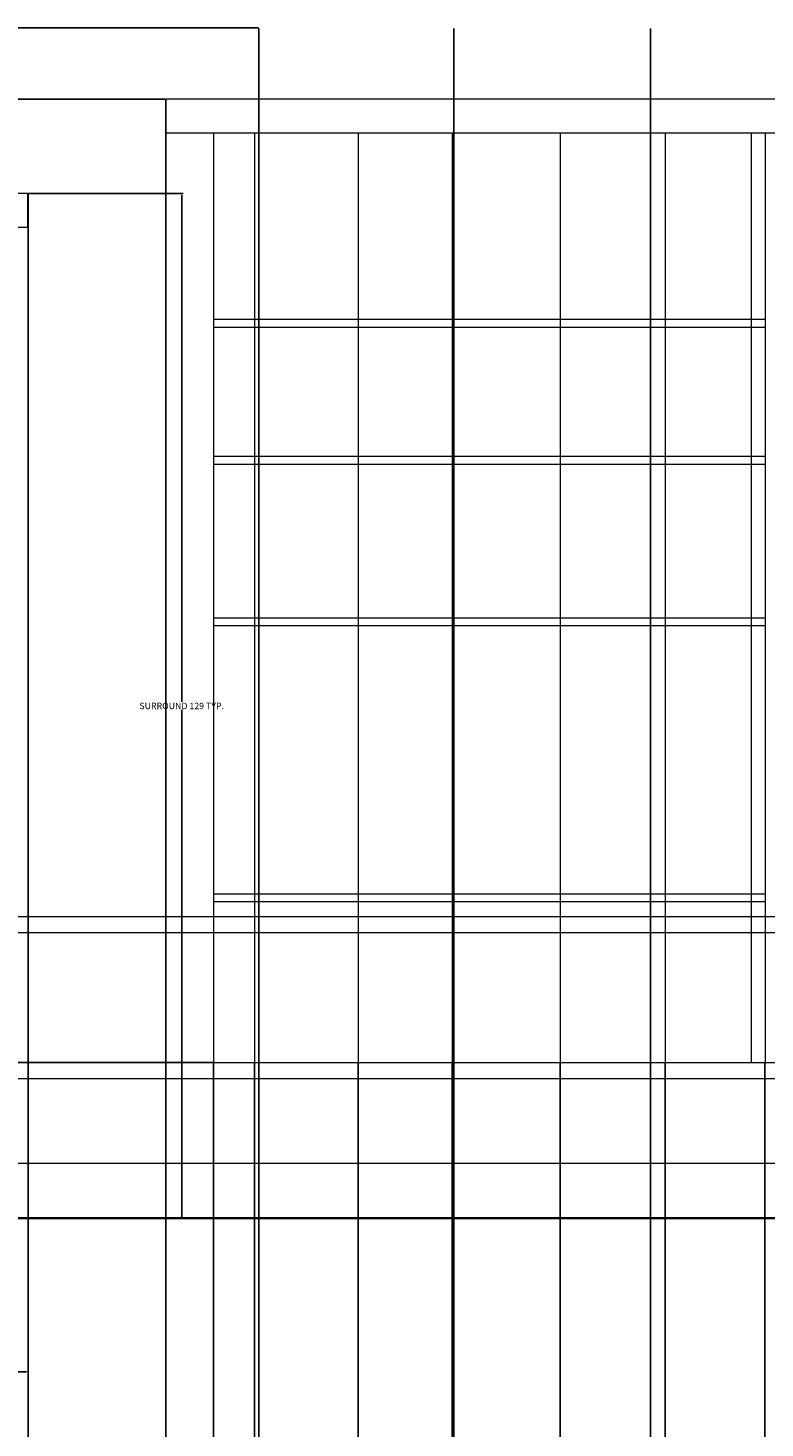
# Model space of a CAD drawing. Units: inches. Extents: x 69 to 650, y -16 to 573.
# Tile 14 of 26: x 290 to 383, y 218 to 394. Entities that reach past the tile are written whole.
import ezdxf

# ---------------------------------------------------------------- set-up
doc = ezdxf.new("R2010")
doc.units = ezdxf.units.IN
doc.header["$MEASUREMENT"] = 0
for name, color, linetype, lineweight in [('A-ANNO-DIMS', 2, 'Continuous', 18), ('A-ELEV', 8, 'Continuous', 18), ('A-GLAZ', 4, 'Continuous', 18), ('A-WALL', 7, 'Continuous', 35)]:
    doc.layers.add(name, color=color, linetype=linetype, lineweight=lineweight)
doc.styles.get("Standard").update_dxf_attribs({"font": 'arial.ttf'})
doc.dimstyles.get("Standard").update_dxf_attribs({"dimtxt": 0.8125, "dimasz": 0.18, "dimexe": 0.18, "dimexo": 0.0625, "dimgap": 0.09, "dimtad": 0, "dimtih": 1, "dimtoh": 1, "dimdec": 4, "dimzin": 0, "dimdsep": 46, "dimlunit": 4, "dimtxsty": 'Standard', "dimcen": 0.09, "dimadec": 0, "dimazin": 0, "dimtfac": 1, "dimtdec": 4, "dimtofl": 0, "dimtmove": 0, "dimatfit": 3, "dimfxl": 1, "dimtolj": 1, "dimtzin": 0, "dimarcsym": 0})

# ---------------------------------------------------------------- blocks, each defined once
blk = doc.blocks.new('WIN-ARCH-SURROUND')
for p, q in [((0, 129.06), (0, 124.83)), ((82.63, 129.06), (0, 129.06)), ((82.63, 124.83), (82.63, 129.06)), ((0, 124.83), (82.63, 124.83)), ((2.69, 109.21), (2.69, 124.83)), ((79.05, 109.21), (79.05, 124.83)), ((3.69, 109.21), (2.69, 109.21)), ((3.69, 109.21), (3.69, 105.89)), ((3.69, 109.21), (78.05, 109.21)), ((7.69, 109.21), (7.69, 105.89)), ((8.73, 105.89), (8.73, 109.21)), ((38.31, 109.21), (38.31, 38)), ((40.31, 109.21), (40.31, 38)), ((74.05, 109.21), (74.05, 105.89)), ((78.05, 109.21), (79.05, 109.21)), ((78.05, 109.21), (78.05, 105.89)), ((3.69, 92.64), (3.69, 87.15)), ((7.69, 92.64), (7.69, 87.15)), ((74.05, 92.64), (74.05, 87.15)), ((78.05, 92.64), (78.05, 87.15)), ((3.69, 73.9), (3.69, 69.84)), ((7.69, 73.9), (7.69, 69.84)), ((74.05, 73.9), (74.05, 69.84)), ((78.05, 73.9), (78.05, 69.84)), ((3.69, 56.59), (3.69, 51.51)), ((7.69, 56.59), (7.69, 51.51)), ((74.05, 56.59), (74.05, 51.51)), ((78.05, 56.59), (78.05, 51.51)), ((3.69, 38.26), (3.69, 33.16)), ((7.69, 38.26), (7.69, 33.16)), ((74.05, 38.26), (74.05, 33.16)), ((78.05, 38.26), (78.05, 33.16)), ((3.69, 19.91), (3.69, 0)), ((7.69, 19.91), (7.69, 0)), ((74.05, 19.91), (74.05, 0)), ((78.05, 19.91), (78.05, 0))]:
    blk.add_line(p, q)
for points in [[(8.73, 109.21), (73.05, 109.21), (73.05, 38.26), (8.73, 38.26)], [(9.73, 108.21), (72.05, 108.21), (72.05, 39.26), (9.73, 39.26)], [(2.69, 105.89), (8.73, 105.89), (8.73, 92.64), (2.69, 92.64)], [(73.05, 105.89), (79.1, 105.89), (79.1, 92.64), (73.05, 92.64)], [(2.69, 87.15), (8.73, 87.15), (8.73, 73.9), (2.69, 73.9)], [(73.05, 87.15), (79.1, 87.15), (79.1, 73.9), (73.05, 73.9)], [(2.69, 69.84), (8.73, 69.84), (8.73, 56.59), (2.69, 56.59)], [(73.05, 69.84), (79.1, 69.84), (79.1, 56.59), (73.05, 56.59)], [(2.69, 51.51), (8.73, 51.51), (8.73, 38.26), (2.69, 38.26)], [(73.05, 51.51), (79.1, 51.51), (79.1, 38.26), (73.05, 38.26)], [(2.65, 33.16), (8.69, 33.16), (8.69, 19.91), (2.65, 19.91)], [(73.01, 33.16), (79.06, 33.16), (79.06, 19.91), (73.01, 19.91)]]:
    blk.add_lwpolyline(points, close=True)
blk.add_ellipse((40.89, 109.21), major_axis=(32.16, 0), ratio=0.165597, start_param=6.283185, end_param=9.424778)
blk = doc.blocks.new('*D13')
at = {"layer": 'A-ANNO-DIMS', "color": 0, "lineweight": -2, "transparency": 16777216}
for p, q in [((290.51, 372.99), (309.99, 372.99)), ((309.81, 372.81), (309.81, 308.97)), ((309.81, 244.11), (309.81, 307.95)), ((290.51, 243.93), (309.99, 243.93))]:
    blk.add_line(p, q, dxfattribs=at)
at = {"layer": 'A-ANNO-DIMS', "color": 0, "transparency": 16777216}
for points in [[(309.78, 372.81), (309.84, 372.81), (309.81, 372.99)], [(309.78, 244.11), (309.84, 244.11), (309.81, 243.93)]]:
    blk.add_solid(points, dxfattribs=at)
at = {"layer": 'Defpoints', "color": 0, "transparency": 16777216}
for p in [(290.45, 372.99), (309.81, 372.99), (290.45, 243.93)]:
    blk.add_point(p, dxfattribs=at)
at = {"layer": 'A-ANNO-DIMS', "color": 0, "transparency": 16777216, "insert": (309.81, 308.46), "char_height": 0.8125, "attachment_point": 5}
blk.add_mtext('\\A1;SURROUND 129 TYP.', dxfattribs=at)
blk = doc.blocks.new('*D14')
at = {"layer": 'A-ANNO-DIMS', "color": 0, "lineweight": -2, "transparency": 16777216}
for p, q in [((207.81, 243.87), (207.81, 224.39)), ((290.45, 243.87), (290.45, 224.39)), ((207.99, 224.57), (247.06, 224.57)), ((290.27, 224.57), (251.2, 224.57))]:
    blk.add_line(p, q, dxfattribs=at)
at = {"layer": 'A-ANNO-DIMS', "color": 0, "transparency": 16777216}
for points in [[(207.99, 224.6), (207.99, 224.54), (207.81, 224.57)], [(290.27, 224.6), (290.27, 224.54), (290.45, 224.57)]]:
    blk.add_solid(points, dxfattribs=at)
at = {"layer": 'Defpoints', "color": 0, "transparency": 16777216}
for p in [(207.81, 243.93), (290.45, 243.93), (290.45, 224.57)]:
    blk.add_point(p, dxfattribs=at)
at = {"layer": 'A-ANNO-DIMS', "color": 0, "transparency": 16777216, "insert": (249.13, 224.57), "char_height": 0.8125, "attachment_point": 5}
blk.add_mtext('\\A1;83 TYP.', dxfattribs=at)
blk = doc.blocks.new('*D19')
at = {"layer": 'A-ANNO-DIMS', "color": 0, "lineweight": -2, "transparency": 16777216}
for p, q in [((99.56, 471.72), (99.56, 572.74)), ((99.74, 572.56), (358.57, 572.56)), ((619.38, 572.56), (360.54, 572.56)), ((619.56, 87.99), (619.56, 572.74))]:
    blk.add_line(p, q, dxfattribs=at)
at = {"layer": 'A-ANNO-DIMS', "color": 0, "transparency": 16777216}
for points in [[(99.74, 572.59), (99.74, 572.53), (99.56, 572.56)], [(619.38, 572.59), (619.38, 572.53), (619.56, 572.56)]]:
    blk.add_solid(points, dxfattribs=at)
at = {"layer": 'Defpoints', "color": 0, "transparency": 16777216}
for p in [(619.56, 572.56), (99.56, 471.66), (619.56, 87.93)]:
    blk.add_point(p, dxfattribs=at)
at = {"layer": 'A-ANNO-DIMS', "color": 0, "transparency": 16777216, "insert": (359.56, 572.56), "char_height": 0.812, "attachment_point": 5}
blk.add_mtext('\\A1;520', dxfattribs=at)
blk = doc.blocks.new('*D25')
at = {"layer": 'A-ANNO-DIMS', "color": 0, "lineweight": -2, "transparency": 16777216}
for p, q in [((99.49, 243.93), (70.98, 243.93)), ((71.16, 243.75), (71.16, 228.3)), ((71.16, 211.83), (71.16, 227.29)), ((441.88, 211.65), (70.98, 211.65))]:
    blk.add_line(p, q, dxfattribs=at)
at = {"layer": 'A-ANNO-DIMS', "color": 0, "transparency": 16777216}
for points in [[(71.13, 243.75), (71.19, 243.75), (71.16, 243.93)], [(71.13, 211.83), (71.19, 211.83), (71.16, 211.65)]]:
    blk.add_solid(points, dxfattribs=at)
at = {"layer": 'Defpoints', "color": 0, "transparency": 16777216}
for p in [(71.16, 243.93), (99.56, 243.93), (441.94, 211.65)]:
    blk.add_point(p, dxfattribs=at)
at = {"layer": 'A-ANNO-DIMS', "color": 0, "transparency": 16777216, "insert": (71.16, 227.79), "char_height": 0.812, "attachment_point": 5}
blk.add_mtext('\\A1;32.28', dxfattribs=at)
blk = doc.blocks.new('*D37')
at = {"layer": 'A-ANNO-DIMS', "color": 0, "lineweight": -2, "transparency": 16777216}
for p, q in [((307.8, 384.84), (307.8, 35.35)), ((290.45, 372.93), (290.45, 35.35)), ((290.63, 35.53), (297.7, 35.53)), ((307.62, 35.53), (300.55, 35.53))]:
    blk.add_line(p, q, dxfattribs=at)
at = {"layer": 'A-ANNO-DIMS', "color": 0, "transparency": 16777216}
for points in [[(290.63, 35.56), (290.63, 35.5), (290.45, 35.53)], [(307.62, 35.56), (307.62, 35.5), (307.8, 35.53)]]:
    blk.add_solid(points, dxfattribs=at)
at = {"layer": 'Defpoints', "color": 0, "transparency": 16777216}
for p in [(307.8, 384.9), (290.45, 372.99), (307.8, 35.53)]:
    blk.add_point(p, dxfattribs=at)
at = {"layer": 'A-ANNO-DIMS', "color": 0, "transparency": 16777216, "insert": (299.12, 35.53), "char_height": 0.812, "attachment_point": 5}
blk.add_mtext('\\A1;17.35', dxfattribs=at)
blk = doc.blocks.new('*D38')
at = {"layer": 'A-ANNO-DIMS', "color": 0, "lineweight": -2, "transparency": 16777216}
for p, q in [((307.8, 384.84), (307.8, 35.35)), ((390.43, 384.84), (390.43, 35.35)), ((307.98, 35.53), (347.65, 35.53)), ((390.25, 35.53), (350.57, 35.53))]:
    blk.add_line(p, q, dxfattribs=at)
at = {"layer": 'A-ANNO-DIMS', "color": 0, "transparency": 16777216}
for points in [[(307.98, 35.56), (307.98, 35.5), (307.8, 35.53)], [(390.25, 35.56), (390.25, 35.5), (390.43, 35.53)]]:
    blk.add_solid(points, dxfattribs=at)
at = {"layer": 'Defpoints', "color": 0, "transparency": 16777216}
for p in [(307.8, 384.9), (390.43, 384.9), (390.43, 35.53)]:
    blk.add_point(p, dxfattribs=at)
at = {"layer": 'A-ANNO-DIMS', "color": 0, "transparency": 16777216, "insert": (349.11, 35.53), "char_height": 0.812, "attachment_point": 5}
blk.add_mtext('\\A1;82.63', dxfattribs=at)
blk = doc.blocks.new('*D58')
at = {"layer": 'A-ANNO-DIMS', "color": 0, "lineweight": -2, "transparency": 16777216}
for p, q in [((313.74, 263.53), (70.98, 263.53)), ((71.16, 263.35), (71.16, 254.23)), ((71.16, 244.11), (71.16, 253.22)), ((190.24, 243.93), (70.98, 243.93))]:
    blk.add_line(p, q, dxfattribs=at)
at = {"layer": 'A-ANNO-DIMS', "color": 0, "transparency": 16777216}
for points in [[(71.13, 263.35), (71.19, 263.35), (71.16, 263.53)], [(71.13, 244.11), (71.19, 244.11), (71.16, 243.93)]]:
    blk.add_solid(points, dxfattribs=at)
at = {"layer": 'Defpoints', "color": 0, "transparency": 16777216}
for p in [(71.16, 263.53), (313.81, 263.53), (190.3, 243.93)]:
    blk.add_point(p, dxfattribs=at)
at = {"layer": 'A-ANNO-DIMS', "color": 0, "transparency": 16777216, "insert": (71.16, 253.73), "char_height": 0.812, "attachment_point": 5}
blk.add_mtext('\\A1;19.595', dxfattribs=at)
blk = doc.blocks.new('*D59')
at = {"layer": 'A-ANNO-DIMS', "color": 0, "lineweight": -2, "transparency": 16777216}
for p, q in [((214.82, 402.3), (70.98, 402.3)), ((71.16, 402.12), (71.16, 394.11)), ((71.16, 385.08), (71.16, 393.1)), ((307.73, 384.9), (70.98, 384.9))]:
    blk.add_line(p, q, dxfattribs=at)
at = {"layer": 'A-ANNO-DIMS', "color": 0, "transparency": 16777216}
for points in [[(71.13, 402.12), (71.19, 402.12), (71.16, 402.3)], [(71.13, 385.08), (71.19, 385.08), (71.16, 384.9)]]:
    blk.add_solid(points, dxfattribs=at)
at = {"layer": 'Defpoints', "color": 0, "transparency": 16777216}
for p in [(71.16, 402.3), (214.89, 402.3), (307.8, 384.9)]:
    blk.add_point(p, dxfattribs=at)
at = {"layer": 'A-ANNO-DIMS', "color": 0, "transparency": 16777216, "insert": (71.16, 393.6), "char_height": 0.812, "attachment_point": 5}
blk.add_mtext('\\A1;17.406', dxfattribs=at)
blk = doc.blocks.new('*D63')
at = {"layer": 'A-ANNO-DIMS', "color": 0, "lineweight": -2, "transparency": 16777216}
for p, q in [((319.49, 393.86), (70.98, 393.86)), ((71.16, 393.68), (71.16, 389.88)), ((71.16, 385.08), (71.16, 388.87)), ((307.73, 384.9), (70.98, 384.9))]:
    blk.add_line(p, q, dxfattribs=at)
at = {"layer": 'A-ANNO-DIMS', "color": 0, "transparency": 16777216}
for points in [[(71.13, 393.68), (71.19, 393.68), (71.16, 393.86)], [(71.13, 385.08), (71.19, 385.08), (71.16, 384.9)]]:
    blk.add_solid(points, dxfattribs=at)
at = {"layer": 'Defpoints', "color": 0, "transparency": 16777216}
for p in [(71.16, 393.86), (319.55, 393.86), (307.8, 384.9)]:
    blk.add_point(p, dxfattribs=at)
at = {"layer": 'A-ANNO-DIMS', "color": 0, "transparency": 16777216, "insert": (71.16, 389.38), "char_height": 0.812, "attachment_point": 5}
blk.add_mtext('\\A1;8.959', dxfattribs=at)
blk = doc.blocks.new('*D64')
at = {"layer": 'A-ANNO-DIMS', "color": 0, "lineweight": -2, "transparency": 16777216}
for p, q in [((319.55, 393.8), (319.55, 35.35)), ((344.08, 393.8), (344.08, 35.35)), ((319.73, 35.53), (330.35, 35.53)), ((343.9, 35.53), (333.28, 35.53))]:
    blk.add_line(p, q, dxfattribs=at)
at = {"layer": 'A-ANNO-DIMS', "color": 0, "transparency": 16777216}
for points in [[(319.73, 35.56), (319.73, 35.5), (319.55, 35.53)], [(343.9, 35.56), (343.9, 35.5), (344.08, 35.53)]]:
    blk.add_solid(points, dxfattribs=at)
at = {"layer": 'Defpoints', "color": 0, "transparency": 16777216}
for p in [(319.55, 393.86), (344.08, 393.86), (344.08, 35.53)]:
    blk.add_point(p, dxfattribs=at)
at = {"layer": 'A-ANNO-DIMS', "color": 0, "transparency": 16777216, "insert": (331.82, 35.53), "char_height": 0.812, "attachment_point": 5}
blk.add_mtext('\\A1;24.53', dxfattribs=at)
blk = doc.blocks.new('*D65')
at = {"layer": 'A-ANNO-DIMS', "color": 0, "lineweight": -2, "transparency": 16777216}
for p, q in [((344.08, 393.8), (344.08, 35.35)), ((368.88, 393.8), (368.88, 35.35)), ((344.26, 35.53), (355.33, 35.53)), ((368.7, 35.53), (357.63, 35.53))]:
    blk.add_line(p, q, dxfattribs=at)
at = {"layer": 'A-ANNO-DIMS', "color": 0, "transparency": 16777216}
for points in [[(344.26, 35.56), (344.26, 35.5), (344.08, 35.53)], [(368.7, 35.56), (368.7, 35.5), (368.88, 35.53)]]:
    blk.add_solid(points, dxfattribs=at)
at = {"layer": 'Defpoints', "color": 0, "transparency": 16777216}
for p in [(344.08, 393.86), (368.88, 393.86), (368.88, 35.53)]:
    blk.add_point(p, dxfattribs=at)
at = {"layer": 'A-ANNO-DIMS', "color": 0, "transparency": 16777216, "insert": (356.48, 35.53), "char_height": 0.812, "attachment_point": 5}
blk.add_mtext('\\A1;24.8', dxfattribs=at)
blk = doc.blocks.new('*D66')
at = {"layer": 'A-ANNO-DIMS', "color": 0, "lineweight": -2, "transparency": 16777216}
for p, q in [((313.81, 263.46), (313.81, 35.35)), ((318.98, 263.46), (318.98, 35.35)), ((313.99, 35.53), (314.93, 35.53)), ((318.8, 35.53), (317.85, 35.53))]:
    blk.add_line(p, q, dxfattribs=at)
at = {"layer": 'A-ANNO-DIMS', "color": 0, "transparency": 16777216}
for points in [[(313.99, 35.56), (313.99, 35.5), (313.81, 35.53)], [(318.8, 35.56), (318.8, 35.5), (318.98, 35.53)]]:
    blk.add_solid(points, dxfattribs=at)
at = {"layer": 'Defpoints', "color": 0, "transparency": 16777216}
for p in [(313.81, 263.53), (318.98, 263.53), (318.98, 35.53)]:
    blk.add_point(p, dxfattribs=at)
at = {"layer": 'A-ANNO-DIMS', "color": 0, "transparency": 16777216, "insert": (316.39, 35.53), "char_height": 0.812, "attachment_point": 5}
blk.add_mtext('\\A1;5.174', dxfattribs=at)
blk = doc.blocks.new('*D67')
at = {"layer": 'A-ANNO-DIMS', "color": 0, "lineweight": -2, "transparency": 16777216}
for p, q in [((318.98, 263.46), (318.98, 35.35)), ((332.05, 263.46), (332.05, 35.35)), ((319.16, 35.53), (324.09, 35.53)), ((331.87, 35.53), (326.94, 35.53))]:
    blk.add_line(p, q, dxfattribs=at)
at = {"layer": 'A-ANNO-DIMS', "color": 0, "transparency": 16777216}
for points in [[(319.16, 35.56), (319.16, 35.5), (318.98, 35.53)], [(331.87, 35.56), (331.87, 35.5), (332.05, 35.53)]]:
    blk.add_solid(points, dxfattribs=at)
at = {"layer": 'Defpoints', "color": 0, "transparency": 16777216}
for p in [(318.98, 263.53), (332.05, 263.53), (332.05, 35.53)]:
    blk.add_point(p, dxfattribs=at)
at = {"layer": 'A-ANNO-DIMS', "color": 0, "transparency": 16777216, "insert": (325.52, 35.53), "char_height": 0.812, "attachment_point": 5}
blk.add_mtext('\\A1;13.07', dxfattribs=at)
blk = doc.blocks.new('*D68')
at = {"layer": 'A-ANNO-DIMS', "color": 0, "lineweight": -2, "transparency": 16777216}
for p, q in [((332.05, 263.46), (332.05, 35.35)), ((343.89, 263.46), (343.89, 35.35)), ((332.23, 35.53), (336.23, 35.53)), ((343.71, 35.53), (339.71, 35.53))]:
    blk.add_line(p, q, dxfattribs=at)
at = {"layer": 'A-ANNO-DIMS', "color": 0, "transparency": 16777216}
for points in [[(332.23, 35.56), (332.23, 35.5), (332.05, 35.53)], [(343.71, 35.56), (343.71, 35.5), (343.89, 35.53)]]:
    blk.add_solid(points, dxfattribs=at)
at = {"layer": 'Defpoints', "color": 0, "transparency": 16777216}
for p in [(332.05, 263.53), (343.89, 263.53), (343.89, 35.53)]:
    blk.add_point(p, dxfattribs=at)
at = {"layer": 'A-ANNO-DIMS', "color": 0, "transparency": 16777216, "insert": (337.97, 35.53), "char_height": 0.812, "attachment_point": 5}
blk.add_mtext('\\A1;11.839', dxfattribs=at)
blk = doc.blocks.new('*D69')
at = {"layer": 'A-ANNO-DIMS', "color": 0, "lineweight": -2, "transparency": 16777216}
for p, q in [((343.89, 263.46), (343.89, 35.35)), ((357.51, 263.46), (357.51, 35.35)), ((344.07, 35.53), (349.28, 35.53)), ((357.33, 35.53), (352.12, 35.53))]:
    blk.add_line(p, q, dxfattribs=at)
at = {"layer": 'A-ANNO-DIMS', "color": 0, "transparency": 16777216}
for points in [[(344.07, 35.56), (344.07, 35.5), (343.89, 35.53)], [(357.33, 35.56), (357.33, 35.5), (357.51, 35.53)]]:
    blk.add_solid(points, dxfattribs=at)
at = {"layer": 'Defpoints', "color": 0, "transparency": 16777216}
for p in [(343.89, 263.53), (357.51, 263.53), (357.51, 35.53)]:
    blk.add_point(p, dxfattribs=at)
at = {"layer": 'A-ANNO-DIMS', "color": 0, "transparency": 16777216, "insert": (350.7, 35.53), "char_height": 0.812, "attachment_point": 5}
blk.add_mtext('\\A1;13.62', dxfattribs=at)
blk = doc.blocks.new('*D70')
at = {"layer": 'A-ANNO-DIMS', "color": 0, "lineweight": -2, "transparency": 16777216}
for p, q in [((357.51, 263.46), (357.51, 35.35)), ((370.73, 263.46), (370.73, 35.35)), ((357.69, 35.53), (362.46, 35.53)), ((370.55, 35.53), (365.78, 35.53))]:
    blk.add_line(p, q, dxfattribs=at)
at = {"layer": 'A-ANNO-DIMS', "color": 0, "transparency": 16777216}
for points in [[(357.69, 35.56), (357.69, 35.5), (357.51, 35.53)], [(370.55, 35.56), (370.55, 35.5), (370.73, 35.53)]]:
    blk.add_solid(points, dxfattribs=at)
at = {"layer": 'Defpoints', "color": 0, "transparency": 16777216}
for p in [(357.51, 263.53), (370.73, 263.53), (370.73, 35.53)]:
    blk.add_point(p, dxfattribs=at)
at = {"layer": 'A-ANNO-DIMS', "color": 0, "transparency": 16777216, "insert": (364.12, 35.53), "char_height": 0.812, "attachment_point": 5}
blk.add_mtext('\\A1;13.221', dxfattribs=at)
blk = doc.blocks.new('*D71')
at = {"layer": 'A-ANNO-DIMS', "color": 0, "lineweight": -2, "transparency": 16777216}
for p, q in [((370.73, 263.46), (370.73, 35.35)), ((383.3, 263.46), (383.3, 35.35)), ((370.91, 35.53), (375.59, 35.53)), ((383.12, 35.53), (378.44, 35.53))]:
    blk.add_line(p, q, dxfattribs=at)
at = {"layer": 'A-ANNO-DIMS', "color": 0, "transparency": 16777216}
for points in [[(370.91, 35.56), (370.91, 35.5), (370.73, 35.53)], [(383.12, 35.56), (383.12, 35.5), (383.3, 35.53)]]:
    blk.add_solid(points, dxfattribs=at)
at = {"layer": 'Defpoints', "color": 0, "transparency": 16777216}
for p in [(370.73, 263.53), (383.3, 263.53), (383.3, 35.53)]:
    blk.add_point(p, dxfattribs=at)
at = {"layer": 'A-ANNO-DIMS', "color": 0, "transparency": 16777216, "insert": (377.02, 35.53), "char_height": 0.812, "attachment_point": 5}
blk.add_mtext('\\A1;12.57', dxfattribs=at)

msp = doc.modelspace()

# ---------------------------------------------------------------- linework, layer by layer
at = {"layer": 'A-ELEV'}
for p, q in [((190.299, 281.93), (528.812, 281.93)), ((190.299, 279.93), (528.812, 279.93)), ((190.299, 263.5253), (528.812, 263.5253)), ((190.299, 261.5253), (528.812, 261.5253)), ((190.299, 250.8759), (484.5159, 250.8759))]:
    msp.add_line(p, q, dxfattribs=at)
at = {"layer": 'A-GLAZ'}
for p, q in [((390.4291, 384.8986), (307.7955, 384.8986)), ((307.7955, 384.8986), (307.7955, 380.6715)), ((307.7955, 380.6715), (390.4291, 380.6715)), ((313.8067, 380.6715), (313.8067, 263.5253)), ((318.9804, 380.6715), (318.9804, 263.5253)), ((332.0516, 380.6715), (332.0516, 263.5253)), ((343.8902, 380.6715), (343.8902, 263.5253)), ((357.5106, 380.6715), (357.5106, 263.5253)), ((370.7319, 380.6715), (370.7319, 263.5253)), ((381.57, 380.6715), (381.57, 263.5253)), ((383.3022, 380.6715), (383.3022, 263.5253)), ((313.8067, 357.1599), (383.3022, 357.1599)), ((313.8067, 356.1599), (383.3022, 356.1599)), ((313.8067, 339.9061), (383.3022, 339.9061)), ((313.8067, 338.9061), (383.3022, 338.9061)), ((313.8067, 319.5737), (383.3022, 319.5737)), ((313.8067, 318.5737), (383.3022, 318.5737)), ((313.8067, 284.812), (383.3022, 284.812)), ((313.8067, 283.812), (383.3022, 283.812))]:
    msp.add_line(p, q, dxfattribs=at)
at = {"layer": 'A-WALL'}
msp.add_line((99.556, 243.93), (619.555, 243.93), dxfattribs=at)

# ---------------------------------------------------------------- block references
at = {"layer": 'A-GLAZ'}
msp.add_blockref('WIN-ARCH-SURROUND', (207.813, 243.93), dxfattribs=at)

# ---------------------------------------------------------------- dimensions: what is measured, and where the dimension line sits
at = {"layer": 'A-ANNO-DIMS'}
for base, p1, p2, override, picture, middle in [((619.555, 572.5573), (99.556, 471.6595), (619.555, 87.93), {"dimdec": 0, "dimlfac": 1, "dimrnd": 0, "dimzin": 0, "dimdsep": 46, "dimlunit": 2}, '*D19', (359.5555, 572.5573)), ((344.0804, 35.53), (319.5513, 393.8576), (344.0804, 393.8576), {"dimdec": 2, "dimlfac": 1, "dimrnd": 0, "dimzin": 0, "dimdsep": 46, "dimlunit": 2}, '*D64', (331.8159, 35.53)), ((368.881, 35.53), (344.0804, 393.8576), (368.881, 393.8576), {"dimdec": 1, "dimlfac": 1, "dimrnd": 0, "dimzin": 0, "dimdsep": 46, "dimlunit": 2}, '*D65', (356.4807, 35.53)), ((307.7955, 35.53), (290.4461, 372.9907), (307.7955, 384.8986), {"dimdec": 2, "dimlfac": 1, "dimrnd": 0, "dimzin": 0, "dimdsep": 46, "dimlunit": 2}, '*D37', (299.1208, 35.53)), ((390.4291, 35.53), (307.7955, 384.8986), (390.4291, 384.8986), {"dimdec": 2, "dimlfac": 1, "dimrnd": 0, "dimzin": 0, "dimdsep": 46, "dimlunit": 2}, '*D38', (349.1123, 35.53)), ((318.9804, 35.53), (313.8067, 263.5253), (318.9804, 263.5253), {"dimdec": 3, "dimlfac": 1, "dimrnd": 0, "dimzin": 0, "dimdsep": 46, "dimlunit": 2}, '*D66', (316.3936, 35.53)), ((332.0516, 35.53), (318.9804, 263.5253), (332.0516, 263.5253), {"dimdec": 2, "dimlfac": 1, "dimrnd": 0, "dimzin": 0, "dimdsep": 46, "dimlunit": 2}, '*D67', (325.516, 35.53)), ((343.8902, 35.53), (332.0516, 263.5253), (343.8902, 263.5253), {"dimdec": 3, "dimlfac": 1, "dimrnd": 0, "dimzin": 0, "dimdsep": 46, "dimlunit": 2}, '*D68', (337.9709, 35.53)), ((357.5106, 35.53), (343.8902, 263.5253), (357.5106, 263.5253), {"dimdec": 2, "dimlfac": 1, "dimrnd": 0, "dimzin": 0, "dimdsep": 46, "dimlunit": 2}, '*D69', (350.7004, 35.53)), ((370.7319, 35.53), (357.5106, 263.5253), (370.7319, 263.5253), {"dimdec": 3, "dimlfac": 1, "dimrnd": 0, "dimzin": 0, "dimdsep": 46, "dimlunit": 2}, '*D70', (364.1213, 35.53)), ((383.3022, 35.53), (370.7319, 263.5253), (383.3022, 263.5253), {"dimdec": 2, "dimlfac": 1, "dimrnd": 0, "dimzin": 0, "dimdsep": 46, "dimlunit": 2}, '*D71', (377.0171, 35.53))]:
    dim = msp.add_linear_dim(base=base, p1=p1, p2=p2, dimstyle='Standard', override=override, dxfattribs=at)
    dim.commit()
    dim.dimension.update_dxf_attribs({"geometry": picture, "text_midpoint": middle})
for base, p1, p2, override, picture, middle in [((71.156, 402.3042), (307.7955, 384.8986), (214.8863, 402.3042), {"dimdec": 3, "dimlfac": 1, "dimrnd": 0, "dimzin": 0, "dimdsep": 46, "dimlunit": 2}, '*D59', (71.156, 393.6014)), ((71.156, 393.8576), (307.7955, 384.8986), (319.5513, 393.8576), {"dimdec": 3, "dimlfac": 1, "dimrnd": 0, "dimzin": 0, "dimdsep": 46, "dimlunit": 2}, '*D63', (71.156, 389.3781)), ((71.156, 263.5253), (190.299, 243.93), (313.8067, 263.5253), {"dimdec": 3, "dimlfac": 1, "dimrnd": 0, "dimzin": 0, "dimdsep": 46, "dimlunit": 2}, '*D58', (71.156, 253.7277)), ((71.156, 243.93), (441.9398, 211.6519), (99.556, 243.93), {"dimdec": 2, "dimlfac": 1, "dimrnd": 0, "dimzin": 0, "dimdsep": 46, "dimlunit": 2}, '*D25', (71.156, 227.7909))]:
    dim = msp.add_linear_dim(base=base, p1=p1, p2=p2, angle=90, dimstyle='Standard', override=override, dxfattribs=at)
    dim.commit()
    dim.dimension.update_dxf_attribs({"geometry": picture, "text_midpoint": middle})
dim = msp.add_linear_dim(base=(309.8052, 372.9907), p1=(290.4461, 243.93), p2=(290.4461, 372.9907), angle=90, text='SURROUND <> TYP.', dimstyle='Standard', override={"dimdec": 0, "dimlfac": 1, "dimrnd": 0, "dimzin": 0, "dimdsep": 46, "dimlunit": 2}, dxfattribs=at)
dim.commit()
dim.dimension.update_dxf_attribs({"geometry": '*D13', "text_midpoint": (309.8052, 308.4604)})
dim = msp.add_linear_dim(base=(290.4461, 224.5709), p1=(207.8126, 243.93), p2=(290.4461, 243.93), text='<> TYP.', dimstyle='Standard', override={"dimdec": 0, "dimlfac": 1, "dimrnd": 0, "dimzin": 0, "dimdsep": 46, "dimlunit": 2}, dxfattribs=at)
dim.commit()
dim.dimension.update_dxf_attribs({"geometry": '*D14', "text_midpoint": (249.1293, 224.5709)})

doc.saveas('drawing.dxf')
